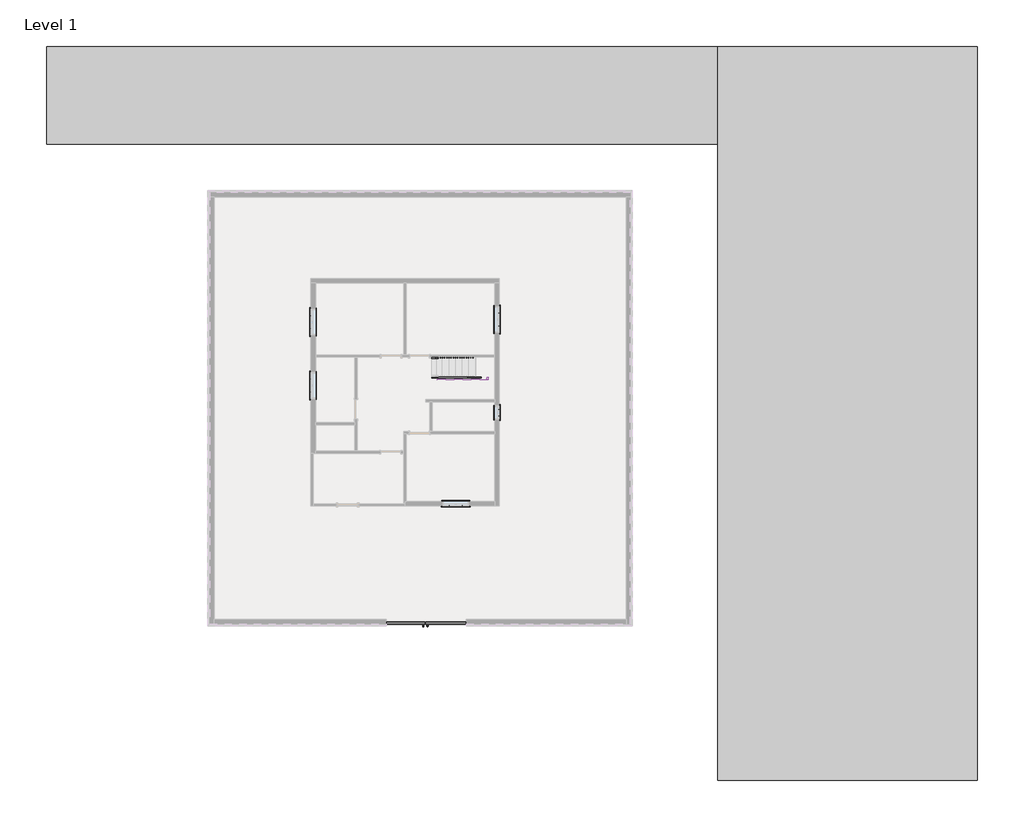
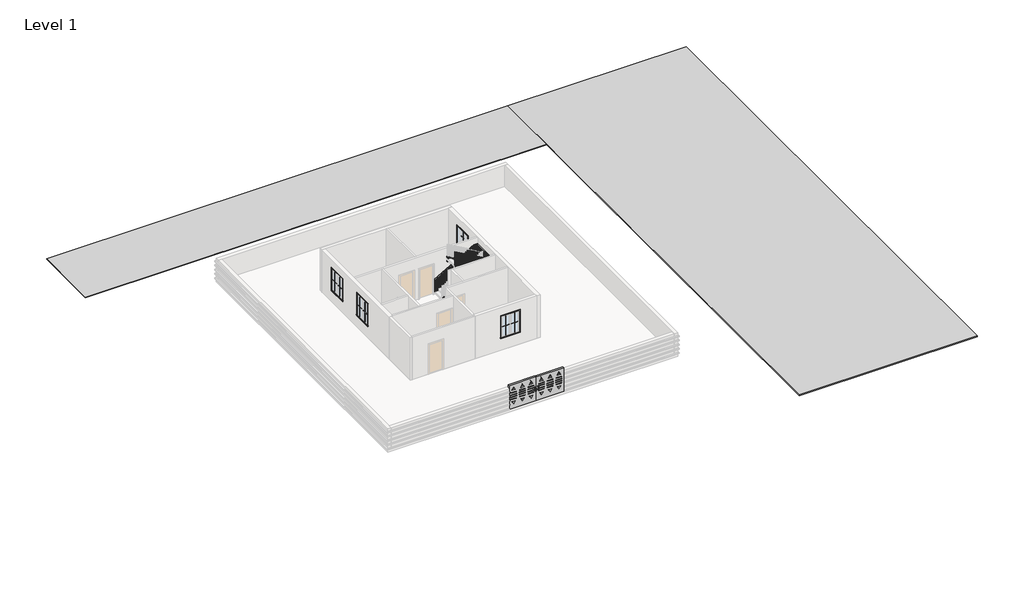
# One storey, part 3 of 3: 22 proxies, 3 members, 1 railing.
"""IFC4 building model written with IfcOpenShell, lengths in millimetres."""

from ifc_helpers import new_model, si_unit, frame, origin, place, context, project, spatial, polyline, outline, extrude, faceted_brep, transform, mapped, element, save
from components import generic_models_afecbd1f, generic_models_1_generic_models_1_28a2cc20, muntin_pattern_2x2_muntin_pattern_2x2_6dad3731, muntin_pattern_2x2_muntin_pattern_2x2_a30a3345, muntin_pattern_2x2_muntin_pattern_2x2_53152e2c, muntin_pattern_2x2_muntin_pattern_2x2_e8f3e573, trim_window_exterior_flat_with_sill_92b9b949, trim_window_exterior_flat_with_sill_a665a915, trim_window_interior_flat_picture_frame_3bb882cf, trim_window_interior_flat_picture_frame_d485c387

model = new_model("IFC4")

# Units and contexts
model_context = context("Model", 3, world=origin())
ifc_project = project(units=[si_unit("LENGTHUNIT", "METRE", prefix="MILLI")], contexts=[model_context])

# Site, building, storey
site = spatial("IfcSite", under=ifc_project)
building = spatial("IfcBuilding", under=site)
storey = spatial("IfcBuildingStorey", under=building, Name="Level 1", Elevation=0.0)

# Proxies
placement = place(None, origin())
generic_models_shape = generic_models_afecbd1f(model_context)
element("IfcBuildingElementProxy", 1, Name="Generic Models", at=placement, inside=storey, context=model_context, shape_type="MappedRepresentation", body=[
    mapped(generic_models_shape, transform((7975.8086384, -3206.75, 0.0), x_axis=(1.0, 0.0, 0.0), y_axis=(0.0, 1.0, 0.0), z_axis=(0.0, 0.0, 1.0))),
])
generic_models_1_generic_models_1_shape = generic_models_1_generic_models_1_28a2cc20(model_context)
element("IfcBuildingElementProxy", 2, Name="Generic Models 1 : Generic Models 1", ObjectType="Generic Models 1 : Generic Models 1", at=placement, inside=storey, context=model_context, shape_type="MappedRepresentation", body=[
    mapped(generic_models_1_generic_models_1_shape, transform((0.0, 0.0, 0.0), x_axis=(1.0, 0.0, 0.0), y_axis=(0.0, 1.0, 0.0), z_axis=(0.0, 0.0, 1.0))),
])
muntin_pattern_2x2_muntin_pattern_2x2_shape = muntin_pattern_2x2_muntin_pattern_2x2_6dad3731(model_context)
element("IfcBuildingElementProxy", 3, Name="Muntin Pattern_2x2 : Muntin Pattern_2x2", ObjectType="Muntin Pattern_2x2 : Muntin Pattern_2x2", at=placement, inside=storey, context=model_context, shape_type="MappedRepresentation", body=[
    mapped(muntin_pattern_2x2_muntin_pattern_2x2_shape, transform((10003.63125, 2232.025, 984.25), x_axis=(-1.0, 0.0, 0.0), y_axis=(0.0, -1.0, 0.0), z_axis=(0.0, 0.0, 1.0))),
])
element("IfcBuildingElementProxy", 4, Name="Muntin Pattern_2x2 : Muntin Pattern_2x2", ObjectType="Muntin Pattern_2x2 : Muntin Pattern_2x2", at=placement, inside=storey, context=model_context, shape_type="MappedRepresentation", body=[
    mapped(muntin_pattern_2x2_muntin_pattern_2x2_shape, transform((2917.825, 7567.6125, 984.25), x_axis=(0.0, 1.0, 0.0), y_axis=(-1.0, 0.0, 0.0), z_axis=(0.0, 0.0, 1.0))),
])
element("IfcBuildingElementProxy", 5, Name="Muntin Pattern_2x2 : Muntin Pattern_2x2", ObjectType="Muntin Pattern_2x2 : Muntin Pattern_2x2", at=placement, inside=storey, context=model_context, shape_type="MappedRepresentation", body=[
    mapped(muntin_pattern_2x2_muntin_pattern_2x2_shape, transform((2917.825, 10536.2375, 984.25), x_axis=(0.0, 1.0, 0.0), y_axis=(-1.0, 0.0, 0.0), z_axis=(0.0, 0.0, 1.0))),
])
element("IfcBuildingElementProxy", 6, Name="Muntin Pattern_2x2 : Muntin Pattern_2x2", ObjectType="Muntin Pattern_2x2 : Muntin Pattern_2x2", at=placement, inside=storey, context=model_context, shape_type="MappedRepresentation", body=[
    mapped(muntin_pattern_2x2_muntin_pattern_2x2_shape, transform((11737.975, 11264.9, 984.25), x_axis=(0.0, -1.0, 0.0), y_axis=(1.0, 0.0, 0.0), z_axis=(0.0, 0.0, 1.0))),
])
muntin_pattern_2x2_muntin_pattern_2x2_2_shape = muntin_pattern_2x2_muntin_pattern_2x2_a30a3345(model_context)
element("IfcBuildingElementProxy", 7, Name="Muntin Pattern_2x2 : Muntin Pattern_2x2", ObjectType="Muntin Pattern_2x2 : Muntin Pattern_2x2", at=placement, inside=storey, context=model_context, shape_type="MappedRepresentation", body=[
    mapped(muntin_pattern_2x2_muntin_pattern_2x2_2_shape, transform((9397.20625, 2232.025, 984.25), x_axis=(1.0, 0.0, 0.0), y_axis=(0.0, 1.0, 0.0), z_axis=(0.0, 0.0, 1.0))),
])
element("IfcBuildingElementProxy", 8, Name="Muntin Pattern_2x2 : Muntin Pattern_2x2", ObjectType="Muntin Pattern_2x2 : Muntin Pattern_2x2", at=placement, inside=storey, context=model_context, shape_type="MappedRepresentation", body=[
    mapped(muntin_pattern_2x2_muntin_pattern_2x2_2_shape, transform((2917.825, 8174.0375, 984.25), x_axis=(0.0, -1.0, 0.0), y_axis=(1.0, 0.0, 0.0), z_axis=(0.0, 0.0, 1.0))),
])
element("IfcBuildingElementProxy", 9, Name="Muntin Pattern_2x2 : Muntin Pattern_2x2", ObjectType="Muntin Pattern_2x2 : Muntin Pattern_2x2", at=placement, inside=storey, context=model_context, shape_type="MappedRepresentation", body=[
    mapped(muntin_pattern_2x2_muntin_pattern_2x2_2_shape, transform((2917.825, 11142.6625, 984.25), x_axis=(0.0, -1.0, 0.0), y_axis=(1.0, 0.0, 0.0), z_axis=(0.0, 0.0, 1.0))),
])
element("IfcBuildingElementProxy", 10, Name="Muntin Pattern_2x2 : Muntin Pattern_2x2", ObjectType="Muntin Pattern_2x2 : Muntin Pattern_2x2", at=placement, inside=storey, context=model_context, shape_type="MappedRepresentation", body=[
    mapped(muntin_pattern_2x2_muntin_pattern_2x2_2_shape, transform((11737.975, 10658.475, 984.25), x_axis=(0.0, 1.0, 0.0), y_axis=(-1.0, 0.0, 0.0), z_axis=(0.0, 0.0, 1.0))),
])
muntin_pattern_2x2_muntin_pattern_2x2_3_shape = muntin_pattern_2x2_muntin_pattern_2x2_53152e2c(model_context)
element("IfcBuildingElementProxy", 11, Name="Muntin Pattern_2x2 : Muntin Pattern_2x2", ObjectType="Muntin Pattern_2x2 : Muntin Pattern_2x2", at=placement, inside=storey, context=model_context, shape_type="MappedRepresentation", body=[
    mapped(muntin_pattern_2x2_muntin_pattern_2x2_3_shape, transform((11737.975, 6748.4625, 984.25), x_axis=(0.0, -1.0, 0.0), y_axis=(1.0, 0.0, 0.0), z_axis=(0.0, 0.0, 1.0))),
])
muntin_pattern_2x2_muntin_pattern_2x2_4_shape = muntin_pattern_2x2_muntin_pattern_2x2_e8f3e573(model_context)
element("IfcBuildingElementProxy", 12, Name="Muntin Pattern_2x2 : Muntin Pattern_2x2", ObjectType="Muntin Pattern_2x2 : Muntin Pattern_2x2", at=placement, inside=storey, context=model_context, shape_type="MappedRepresentation", body=[
    mapped(muntin_pattern_2x2_muntin_pattern_2x2_4_shape, transform((11737.975, 6446.8375, 984.25), x_axis=(0.0, 1.0, 0.0), y_axis=(-1.0, 0.0, 0.0), z_axis=(0.0, 0.0, 1.0))),
])
trim_window_exterior_flat_with_sill_shape = trim_window_exterior_flat_with_sill_92b9b949(model_context)
element("IfcBuildingElementProxy", 13, Name="Trim-Window-Exterior-Flat : with Sill", ObjectType="Trim-Window-Exterior-Flat : with Sill", at=placement, inside=storey, context=model_context, shape_type="MappedRepresentation", body=[
    mapped(trim_window_exterior_flat_with_sill_shape, transform((9700.41875, 2222.5, 2438.4), x_axis=(1.0, 0.0, 0.0), y_axis=(0.0, 0.0, 1.0), z_axis=(0.0, -1.0, 0.0))),
])
element("IfcBuildingElementProxy", 14, Name="Trim-Window-Exterior-Flat : with Sill", ObjectType="Trim-Window-Exterior-Flat : with Sill", at=placement, inside=storey, context=model_context, shape_type="MappedRepresentation", body=[
    mapped(trim_window_exterior_flat_with_sill_shape, transform((2908.3, 7870.825, 2438.4), x_axis=(0.0, -1.0, 0.0), y_axis=(0.0, 0.0, 1.0), z_axis=(-1.0, 0.0, 0.0))),
])
element("IfcBuildingElementProxy", 15, Name="Trim-Window-Exterior-Flat : with Sill", ObjectType="Trim-Window-Exterior-Flat : with Sill", at=placement, inside=storey, context=model_context, shape_type="MappedRepresentation", body=[
    mapped(trim_window_exterior_flat_with_sill_shape, transform((2908.3, 10839.45, 2438.4), x_axis=(0.0, -1.0, 0.0), y_axis=(0.0, 0.0, 1.0), z_axis=(-1.0, 0.0, 0.0))),
])
element("IfcBuildingElementProxy", 16, Name="Trim-Window-Exterior-Flat : with Sill", ObjectType="Trim-Window-Exterior-Flat : with Sill", at=placement, inside=storey, context=model_context, shape_type="MappedRepresentation", body=[
    mapped(trim_window_exterior_flat_with_sill_shape, transform((11747.5, 10961.6875, 2438.4), x_axis=(0.0, 1.0, 0.0), y_axis=(0.0, 0.0, 1.0), z_axis=(1.0, 0.0, 0.0))),
])
trim_window_exterior_flat_with_sill_2_shape = trim_window_exterior_flat_with_sill_a665a915(model_context)
element("IfcBuildingElementProxy", 17, Name="Trim-Window-Exterior-Flat : with Sill", ObjectType="Trim-Window-Exterior-Flat : with Sill", at=placement, inside=storey, context=model_context, shape_type="MappedRepresentation", body=[
    mapped(trim_window_exterior_flat_with_sill_2_shape, transform((11747.5, 6597.65, 1828.8), x_axis=(0.0, 1.0, 0.0), y_axis=(0.0, 0.0, 1.0), z_axis=(1.0, 0.0, 0.0))),
])
trim_window_interior_flat_picture_frame_shape = trim_window_interior_flat_picture_frame_3bb882cf(model_context)
element("IfcBuildingElementProxy", 18, Name="Trim-Window-Interior-Flat : Picture Frame", ObjectType="Trim-Window-Interior-Flat : Picture Frame", at=placement, inside=storey, context=model_context, shape_type="MappedRepresentation", body=[
    mapped(trim_window_interior_flat_picture_frame_shape, transform((9700.41875, 2451.1, 2438.4), x_axis=(-1.0, 0.0, 0.0), y_axis=(0.0, 0.0, 1.0), z_axis=(0.0, 1.0, 0.0))),
])
element("IfcBuildingElementProxy", 19, Name="Trim-Window-Interior-Flat : Picture Frame", ObjectType="Trim-Window-Interior-Flat : Picture Frame", at=placement, inside=storey, context=model_context, shape_type="MappedRepresentation", body=[
    mapped(trim_window_interior_flat_picture_frame_shape, transform((3136.9, 7870.825, 2438.4), x_axis=(0.0, 1.0, 0.0), y_axis=(0.0, 0.0, 1.0), z_axis=(1.0, 0.0, 0.0))),
])
element("IfcBuildingElementProxy", 20, Name="Trim-Window-Interior-Flat : Picture Frame", ObjectType="Trim-Window-Interior-Flat : Picture Frame", at=placement, inside=storey, context=model_context, shape_type="MappedRepresentation", body=[
    mapped(trim_window_interior_flat_picture_frame_shape, transform((3136.9, 10839.45, 2438.4), x_axis=(0.0, 1.0, 0.0), y_axis=(0.0, 0.0, 1.0), z_axis=(1.0, 0.0, 0.0))),
])
element("IfcBuildingElementProxy", 21, Name="Trim-Window-Interior-Flat : Picture Frame", ObjectType="Trim-Window-Interior-Flat : Picture Frame", at=placement, inside=storey, context=model_context, shape_type="MappedRepresentation", body=[
    mapped(trim_window_interior_flat_picture_frame_shape, transform((11518.9, 10961.6875, 2438.4), x_axis=(0.0, -1.0, 0.0), y_axis=(0.0, 0.0, 1.0), z_axis=(-1.0, 0.0, 0.0))),
])
trim_window_interior_flat_picture_frame_2_shape = trim_window_interior_flat_picture_frame_d485c387(model_context)
element("IfcBuildingElementProxy", 22, Name="Trim-Window-Interior-Flat : Picture Frame", ObjectType="Trim-Window-Interior-Flat : Picture Frame", at=placement, inside=storey, context=model_context, shape_type="MappedRepresentation", body=[
    mapped(trim_window_interior_flat_picture_frame_2_shape, transform((11518.9, 6597.65, 1828.8), x_axis=(0.0, -1.0, 0.0), y_axis=(0.0, 0.0, 1.0), z_axis=(-1.0, 0.0, 0.0))),
])

# Members
element("IfcMember", 23, ObjectType="Stringer - 2\" Width", at=placement, inside=storey, context=model_context, shape_type="SweptSolid", body=[
    extrude(outline(polyline([(249.0972589, 8572.5), (0.0, 8572.5), (0.0, 8751.427498), (1354.0336853, 11163.3), (1703.5814695, 11163.3), (249.0972589, 8572.5)])), frame((0.0, 8229.6, 0.0), z_axis=(0.0, 1.0, 0.0), x_axis=(0.0, 0.0, 1.0)), (0.0, 0.0, 1.0), 50.8),
])
element("IfcMember", 24, ObjectType="Stringer - 2\" Width", at=placement, inside=storey, context=model_context, shape_type="SweptSolid", body=[
    extrude(outline(polyline([(11163.3, 8280.4), (11214.1, 8280.4), (11214.1, 8178.8), (11163.3, 8178.8), (11163.3, 8280.4)])), frame((0.0, 0.0, 1464.7333333), z_axis=(0.0, 0.0, 1.0), x_axis=(1.0, 0.0, 0.0)), (0.0, 0.0, 1.0), 304.8),
])
element("IfcMember", 25, ObjectType="Stringer - 2\" Width", at=placement, inside=storey, context=model_context, shape_type="SweptSolid", body=[
    extrude(outline(polyline([(1552.253054, 11214.1), (1900.9317281, 11214.1), (3227.3761726, 8826.5), (2878.6974984, 8826.5), (1552.253054, 11214.1)])), frame((0.0, 8128.0, 0.0), z_axis=(0.0, 1.0, 0.0), x_axis=(0.0, 0.0, 1.0)), (0.0, 0.0, 1.0), 50.8),
])

# Railing
element("IfcRailing", 26, ObjectType="Handrail - Rectangular", at=placement, inside=storey, context=model_context, shape_type="SolidModel", body=[
    faceted_brep([(8572.5, 9194.8, 1083.7333333), (8572.5, 9194.8, 1025.0853937), (8572.5, 9144.0, 1025.0853937), (8572.5, 9144.0, 1083.7333333), (11214.1, 9194.8, 2607.7333333), (11227.7030954, 9194.8, 2556.9333333), (11227.7030954, 9144.0, 2556.9333333), (11214.1, 9144.0, 2607.7333333), (11518.9, 9194.8, 2607.7333333), (11518.9, 9194.8, 2556.9333333), (11468.1, 9144.0, 2556.9333333), (11468.1, 9144.0, 2607.7333333), (11518.9, 7340.6, 2607.7333333), (11518.9, 7289.8, 2556.9333333), (11468.1, 7289.8, 2556.9333333), (11468.1, 7340.6, 2607.7333333), (11518.9, 7340.6, 2676.187234), (11518.9, 7289.8, 2625.387234), (11468.1, 7289.8, 2625.387234), (11468.1, 7340.6, 2676.187234), (11518.9, 7213.6, 2676.187234), (11518.9, 7213.6, 2625.387234), (11468.1, 7264.4, 2625.387234), (11468.1, 7264.4, 2676.187234), (11391.9, 7213.6, 2676.187234), (11378.4925101, 7213.6, 2625.387234), (11378.4925101, 7264.4, 2625.387234), (11391.9, 7264.4, 2676.187234), (8826.5, 7213.6, 4131.7333333), (8826.5, 7264.4, 4131.7333333), (8826.5, 7264.4, 4073.3262469), (8826.5, 7213.6, 4073.3262469)], [[[0, 1, 2, 3]], [[1, 0, 4, 5]], [[2, 1, 5, 6]], [[3, 2, 6, 7]], [[0, 3, 7, 4]], [[5, 4, 8, 9]], [[6, 5, 9, 10]], [[7, 6, 10, 11]], [[4, 7, 11, 8]], [[9, 8, 12, 13]], [[10, 9, 13, 14]], [[11, 10, 14, 15]], [[8, 11, 15, 12]], [[13, 12, 16, 17]], [[14, 13, 17, 18]], [[15, 14, 18, 19]], [[12, 15, 19, 16]], [[17, 16, 20, 21]], [[18, 17, 21, 22]], [[19, 18, 22, 23]], [[16, 19, 23, 20]], [[21, 20, 24, 25]], [[22, 21, 25, 26]], [[23, 22, 26, 27]], [[20, 23, 27, 24]], [[28, 29, 30, 31]], [[25, 24, 28, 31]], [[26, 25, 31, 30]], [[27, 26, 30, 29]], [[24, 27, 29, 28]]]),
    extrude(outline(polyline([(4064.3191547, 8842.375), (3048.0, 8842.375), (3048.0, 8861.425), (4053.510644, 8861.425), (4064.3191547, 8842.375)])), frame((0.0, 7229.475, 0.0), z_axis=(0.0, 1.0, 0.0), x_axis=(0.0, 0.0, 1.0)), (0.0, 0.0, 1.0), 19.05),
    extrude(outline(polyline([(4006.6737646, 8943.975), (3048.0, 8943.975), (3048.0, 8963.025), (3995.865254, 8963.025), (4006.6737646, 8943.975)])), frame((0.0, 7229.475, 0.0), z_axis=(0.0, 1.0, 0.0), x_axis=(0.0, 0.0, 1.0)), (0.0, 0.0, 1.0), 19.05),
    extrude(outline(polyline([(3949.0283745, 9045.575), (3048.0, 9045.575), (3048.0, 9064.625), (3938.2198639, 9064.625), (3949.0283745, 9045.575)])), frame((0.0, 7229.475, 0.0), z_axis=(0.0, 1.0, 0.0), x_axis=(0.0, 0.0, 1.0)), (0.0, 0.0, 1.0), 19.05),
    extrude(outline(polyline([(3891.3829845, 9147.175), (2878.6666667, 9147.175), (2878.6666667, 9166.225), (3880.5744738, 9166.225), (3891.3829845, 9147.175)])), frame((0.0, 7229.475, 0.0), z_axis=(0.0, 1.0, 0.0), x_axis=(0.0, 0.0, 1.0)), (0.0, 0.0, 1.0), 19.05),
    extrude(outline(polyline([(3833.7375944, 9248.775), (2878.6666667, 9248.775), (2878.6666667, 9267.825), (3822.9290837, 9267.825), (3833.7375944, 9248.775)])), frame((0.0, 7229.475, 0.0), z_axis=(0.0, 1.0, 0.0), x_axis=(0.0, 0.0, 1.0)), (0.0, 0.0, 1.0), 19.05),
    extrude(outline(polyline([(3776.0922043, 9350.375), (2878.6666667, 9350.375), (2878.6666667, 9369.425), (3765.2836937, 9369.425), (3776.0922043, 9350.375)])), frame((0.0, 7229.475, 0.0), z_axis=(0.0, 1.0, 0.0), x_axis=(0.0, 0.0, 1.0)), (0.0, 0.0, 1.0), 19.05),
    extrude(outline(polyline([(3718.4468142, 9451.975), (2709.3333333, 9451.975), (2709.3333333, 9471.025), (3707.6383036, 9471.025), (3718.4468142, 9451.975)])), frame((0.0, 7229.475, 0.0), z_axis=(0.0, 1.0, 0.0), x_axis=(0.0, 0.0, 1.0)), (0.0, 0.0, 1.0), 19.05),
    extrude(outline(polyline([(3660.8014242, 9553.575), (2709.3333333, 9553.575), (2709.3333333, 9572.625), (3649.9929135, 9572.625), (3660.8014242, 9553.575)])), frame((0.0, 7229.475, 0.0), z_axis=(0.0, 1.0, 0.0), x_axis=(0.0, 0.0, 1.0)), (0.0, 0.0, 1.0), 19.05),
    extrude(outline(polyline([(3603.1446885, 9655.175), (2709.3333333, 9655.175), (2709.3333333, 9674.225), (3592.1543039, 9674.225), (3603.1446885, 9655.175)])), frame((0.0, 7229.475, 0.0), z_axis=(0.0, 1.0, 0.0), x_axis=(0.0, 0.0, 1.0)), (0.0, 0.0, 1.0), 19.05),
    extrude(outline(polyline([(3545.510644, 9756.775), (2540.0, 9756.775), (2540.0, 9775.825), (3534.7021334, 9775.825), (3545.510644, 9756.775)])), frame((0.0, 7229.475, 0.0), z_axis=(0.0, 1.0, 0.0), x_axis=(0.0, 0.0, 1.0)), (0.0, 0.0, 1.0), 19.05),
    extrude(outline(polyline([(3487.865254, 9858.375), (2540.0, 9858.375), (2540.0, 9877.425), (3477.0567433, 9877.425), (3487.865254, 9858.375)])), frame((0.0, 7229.475, 0.0), z_axis=(0.0, 1.0, 0.0), x_axis=(0.0, 0.0, 1.0)), (0.0, 0.0, 1.0), 19.05),
    extrude(outline(polyline([(3430.2198639, 9959.975), (2540.0, 9959.975), (2540.0, 9979.025), (3419.4113533, 9979.025), (3430.2198639, 9959.975)])), frame((0.0, 7229.475, 0.0), z_axis=(0.0, 1.0, 0.0), x_axis=(0.0, 0.0, 1.0)), (0.0, 0.0, 1.0), 19.05),
    extrude(outline(polyline([(3372.5744738, 10061.575), (2370.6666667, 10061.575), (2370.6666667, 10080.625), (3361.7659632, 10080.625), (3372.5744738, 10061.575)])), frame((0.0, 7229.475, 0.0), z_axis=(0.0, 1.0, 0.0), x_axis=(0.0, 0.0, 1.0)), (0.0, 0.0, 1.0), 19.05),
    extrude(outline(polyline([(3314.9290837, 10163.175), (2370.6666667, 10163.175), (2370.6666667, 10182.225), (3304.1205731, 10182.225), (3314.9290837, 10163.175)])), frame((0.0, 7229.475, 0.0), z_axis=(0.0, 1.0, 0.0), x_axis=(0.0, 0.0, 1.0)), (0.0, 0.0, 1.0), 19.05),
    extrude(outline(polyline([(3257.2836937, 10264.775), (2370.6666667, 10264.775), (2370.6666667, 10283.825), (3246.475183, 10283.825), (3257.2836937, 10264.775)])), frame((0.0, 7229.475, 0.0), z_axis=(0.0, 1.0, 0.0), x_axis=(0.0, 0.0, 1.0)), (0.0, 0.0, 1.0), 19.05),
    extrude(outline(polyline([(3199.6383036, 10366.375), (2201.3333333, 10366.375), (2201.3333333, 10385.425), (3188.829793, 10385.425), (3199.6383036, 10366.375)])), frame((0.0, 7229.475, 0.0), z_axis=(0.0, 1.0, 0.0), x_axis=(0.0, 0.0, 1.0)), (0.0, 0.0, 1.0), 19.05),
    extrude(outline(polyline([(3141.9929135, 10467.975), (2201.3333333, 10467.975), (2201.3333333, 10487.025), (3131.1844029, 10487.025), (3141.9929135, 10467.975)])), frame((0.0, 7229.475, 0.0), z_axis=(0.0, 1.0, 0.0), x_axis=(0.0, 0.0, 1.0)), (0.0, 0.0, 1.0), 19.05),
    extrude(outline(polyline([(3084.3475235, 10569.575), (2201.3333333, 10569.575), (2201.3333333, 10588.625), (3073.5390128, 10588.625), (3084.3475235, 10569.575)])), frame((0.0, 7229.475, 0.0), z_axis=(0.0, 1.0, 0.0), x_axis=(0.0, 0.0, 1.0)), (0.0, 0.0, 1.0), 19.05),
    extrude(outline(polyline([(3026.7021334, 10671.175), (2032.0, 10671.175), (2032.0, 10690.225), (3015.8936228, 10690.225), (3026.7021334, 10671.175)])), frame((0.0, 7229.475, 0.0), z_axis=(0.0, 1.0, 0.0), x_axis=(0.0, 0.0, 1.0)), (0.0, 0.0, 1.0), 19.05),
    extrude(outline(polyline([(2969.0567433, 10772.775), (2032.0, 10772.775), (2032.0, 10791.825), (2958.2482327, 10791.825), (2969.0567433, 10772.775)])), frame((0.0, 7229.475, 0.0), z_axis=(0.0, 1.0, 0.0), x_axis=(0.0, 0.0, 1.0)), (0.0, 0.0, 1.0), 19.05),
    extrude(outline(polyline([(2911.4113533, 10874.375), (2032.0, 10874.375), (2032.0, 10893.425), (2900.6028426, 10893.425), (2911.4113533, 10874.375)])), frame((0.0, 7229.475, 0.0), z_axis=(0.0, 1.0, 0.0), x_axis=(0.0, 0.0, 1.0)), (0.0, 0.0, 1.0), 19.05),
    extrude(outline(polyline([(2853.7659632, 10975.975), (1862.6666667, 10975.975), (1862.6666667, 10995.025), (2842.9574525, 10995.025), (2853.7659632, 10975.975)])), frame((0.0, 7229.475, 0.0), z_axis=(0.0, 1.0, 0.0), x_axis=(0.0, 0.0, 1.0)), (0.0, 0.0, 1.0), 19.05),
    extrude(outline(polyline([(2796.1205731, 11077.575), (1862.6666667, 11077.575), (1862.6666667, 11096.625), (2785.3120625, 11096.625), (2796.1205731, 11077.575)])), frame((0.0, 7229.475, 0.0), z_axis=(0.0, 1.0, 0.0), x_axis=(0.0, 0.0, 1.0)), (0.0, 0.0, 1.0), 19.05),
    extrude(outline(polyline([(2738.475183, 11179.175), (1862.6666667, 11179.175), (1862.6666667, 11198.225), (2727.6666724, 11198.225), (2738.475183, 11179.175)])), frame((0.0, 7229.475, 0.0), z_axis=(0.0, 1.0, 0.0), x_axis=(0.0, 0.0, 1.0)), (0.0, 0.0, 1.0), 19.05),
    extrude(outline(polyline([(2680.829793, 11280.775), (1693.3333333, 11280.775), (1693.3333333, 11299.825), (2670.0212823, 11299.825), (2680.829793, 11280.775)])), frame((0.0, 7229.475, 0.0), z_axis=(0.0, 1.0, 0.0), x_axis=(0.0, 0.0, 1.0)), (0.0, 0.0, 1.0), 19.05),
    extrude(outline(polyline([(2623.1844029, 11382.375), (1693.3333333, 11382.375), (1693.3333333, 11401.425), (2612.3758923, 11401.425), (2623.1844029, 11382.375)])), frame((0.0, 7229.475, 0.0), z_axis=(0.0, 1.0, 0.0), x_axis=(0.0, 0.0, 1.0)), (0.0, 0.0, 1.0), 19.05),
    extrude(outline(polyline([(11503.025, 7350.125), (11503.025, 7331.075), (11483.975, 7331.075), (11483.975, 7350.125), (11503.025, 7350.125)])), frame((0.0, 0.0, 1693.3333333), z_axis=(0.0, 0.0, 1.0), x_axis=(1.0, 0.0, 0.0)), (0.0, 0.0, 1.0), 863.6),
    extrude(outline(polyline([(11503.025, 7451.725), (11503.025, 7432.675), (11483.975, 7432.675), (11483.975, 7451.725), (11503.025, 7451.725)])), frame((0.0, 0.0, 1693.3333333), z_axis=(0.0, 0.0, 1.0), x_axis=(1.0, 0.0, 0.0)), (0.0, 0.0, 1.0), 863.6),
    extrude(outline(polyline([(11503.025, 7553.325), (11503.025, 7534.275), (11483.975, 7534.275), (11483.975, 7553.325), (11503.025, 7553.325)])), frame((0.0, 0.0, 1693.3333333), z_axis=(0.0, 0.0, 1.0), x_axis=(1.0, 0.0, 0.0)), (0.0, 0.0, 1.0), 863.6),
    extrude(outline(polyline([(11503.025, 7654.925), (11503.025, 7635.875), (11483.975, 7635.875), (11483.975, 7654.925), (11503.025, 7654.925)])), frame((0.0, 0.0, 1693.3333333), z_axis=(0.0, 0.0, 1.0), x_axis=(1.0, 0.0, 0.0)), (0.0, 0.0, 1.0), 863.6),
    extrude(outline(polyline([(11503.025, 7756.525), (11503.025, 7737.475), (11483.975, 7737.475), (11483.975, 7756.525), (11503.025, 7756.525)])), frame((0.0, 0.0, 1693.3333333), z_axis=(0.0, 0.0, 1.0), x_axis=(1.0, 0.0, 0.0)), (0.0, 0.0, 1.0), 863.6),
    extrude(outline(polyline([(11503.025, 7858.125), (11503.025, 7839.075), (11483.975, 7839.075), (11483.975, 7858.125), (11503.025, 7858.125)])), frame((0.0, 0.0, 1693.3333333), z_axis=(0.0, 0.0, 1.0), x_axis=(1.0, 0.0, 0.0)), (0.0, 0.0, 1.0), 863.6),
    extrude(outline(polyline([(11503.025, 7959.725), (11503.025, 7940.675), (11483.975, 7940.675), (11483.975, 7959.725), (11503.025, 7959.725)])), frame((0.0, 0.0, 1693.3333333), z_axis=(0.0, 0.0, 1.0), x_axis=(1.0, 0.0, 0.0)), (0.0, 0.0, 1.0), 863.6),
    extrude(outline(polyline([(11503.025, 8061.325), (11503.025, 8042.275), (11483.975, 8042.275), (11483.975, 8061.325), (11503.025, 8061.325)])), frame((0.0, 0.0, 1693.3333333), z_axis=(0.0, 0.0, 1.0), x_axis=(1.0, 0.0, 0.0)), (0.0, 0.0, 1.0), 863.6),
    extrude(outline(polyline([(11503.025, 8162.925), (11503.025, 8143.875), (11483.975, 8143.875), (11483.975, 8162.925), (11503.025, 8162.925)])), frame((0.0, 0.0, 1693.3333333), z_axis=(0.0, 0.0, 1.0), x_axis=(1.0, 0.0, 0.0)), (0.0, 0.0, 1.0), 863.6),
    extrude(outline(polyline([(11503.025, 8264.525), (11503.025, 8245.475), (11483.975, 8245.475), (11483.975, 8264.525), (11503.025, 8264.525)])), frame((0.0, 0.0, 1693.3333333), z_axis=(0.0, 0.0, 1.0), x_axis=(1.0, 0.0, 0.0)), (0.0, 0.0, 1.0), 863.6),
    extrude(outline(polyline([(11503.025, 8366.125), (11503.025, 8347.075), (11483.975, 8347.075), (11483.975, 8366.125), (11503.025, 8366.125)])), frame((0.0, 0.0, 1693.3333333), z_axis=(0.0, 0.0, 1.0), x_axis=(1.0, 0.0, 0.0)), (0.0, 0.0, 1.0), 863.6),
    extrude(outline(polyline([(11503.025, 8467.725), (11503.025, 8448.675), (11483.975, 8448.675), (11483.975, 8467.725), (11503.025, 8467.725)])), frame((0.0, 0.0, 1693.3333333), z_axis=(0.0, 0.0, 1.0), x_axis=(1.0, 0.0, 0.0)), (0.0, 0.0, 1.0), 863.6),
    extrude(outline(polyline([(11503.025, 8569.325), (11503.025, 8550.275), (11483.975, 8550.275), (11483.975, 8569.325), (11503.025, 8569.325)])), frame((0.0, 0.0, 1693.3333333), z_axis=(0.0, 0.0, 1.0), x_axis=(1.0, 0.0, 0.0)), (0.0, 0.0, 1.0), 863.6),
    extrude(outline(polyline([(11503.025, 8670.925), (11503.025, 8651.875), (11483.975, 8651.875), (11483.975, 8670.925), (11503.025, 8670.925)])), frame((0.0, 0.0, 1693.3333333), z_axis=(0.0, 0.0, 1.0), x_axis=(1.0, 0.0, 0.0)), (0.0, 0.0, 1.0), 863.6),
    extrude(outline(polyline([(11503.025, 8772.525), (11503.025, 8753.475), (11483.975, 8753.475), (11483.975, 8772.525), (11503.025, 8772.525)])), frame((0.0, 0.0, 1693.3333333), z_axis=(0.0, 0.0, 1.0), x_axis=(1.0, 0.0, 0.0)), (0.0, 0.0, 1.0), 863.6),
    extrude(outline(polyline([(11503.025, 8874.125), (11503.025, 8855.075), (11483.975, 8855.075), (11483.975, 8874.125), (11503.025, 8874.125)])), frame((0.0, 0.0, 1693.3333333), z_axis=(0.0, 0.0, 1.0), x_axis=(1.0, 0.0, 0.0)), (0.0, 0.0, 1.0), 863.6),
    extrude(outline(polyline([(11503.025, 8975.725), (11503.025, 8956.675), (11483.975, 8956.675), (11483.975, 8975.725), (11503.025, 8975.725)])), frame((0.0, 0.0, 1693.3333333), z_axis=(0.0, 0.0, 1.0), x_axis=(1.0, 0.0, 0.0)), (0.0, 0.0, 1.0), 863.6),
    extrude(outline(polyline([(11503.025, 9077.325), (11503.025, 9058.275), (11483.975, 9058.275), (11483.975, 9077.325), (11503.025, 9077.325)])), frame((0.0, 0.0, 1693.3333333), z_axis=(0.0, 0.0, 1.0), x_axis=(1.0, 0.0, 0.0)), (0.0, 0.0, 1.0), 863.6),
    extrude(outline(polyline([(11407.775, 9178.925), (11426.825, 9178.925), (11426.825, 9159.875), (11407.775, 9159.875), (11407.775, 9178.925)])), frame((0.0, 0.0, 1693.3333333), z_axis=(0.0, 0.0, 1.0), x_axis=(1.0, 0.0, 0.0)), (0.0, 0.0, 1.0), 863.6),
    extrude(outline(polyline([(11306.175, 9178.925), (11325.225, 9178.925), (11325.225, 9159.875), (11306.175, 9159.875), (11306.175, 9178.925)])), frame((0.0, 0.0, 1693.3333333), z_axis=(0.0, 0.0, 1.0), x_axis=(1.0, 0.0, 0.0)), (0.0, 0.0, 1.0), 863.6),
    extrude(outline(polyline([(2543.5902013, 11204.575), (1693.3333333, 11204.575), (1693.3333333, 11223.625), (2554.580586, 11223.625), (2543.5902013, 11204.575)])), frame((0.0, 9159.875, 0.0), z_axis=(0.0, 1.0, 0.0), x_axis=(0.0, 0.0, 1.0)), (0.0, 0.0, 1.0), 19.05),
    extrude(outline(polyline([(2484.9748167, 11102.975), (1524.0, 11102.975), (1524.0, 11122.025), (2495.9652013, 11122.025), (2484.9748167, 11102.975)])), frame((0.0, 9159.875, 0.0), z_axis=(0.0, 1.0, 0.0), x_axis=(0.0, 0.0, 1.0)), (0.0, 0.0, 1.0), 19.05),
    extrude(outline(polyline([(2426.3594321, 11001.375), (1524.0, 11001.375), (1524.0, 11020.425), (2437.3498167, 11020.425), (2426.3594321, 11001.375)])), frame((0.0, 9159.875, 0.0), z_axis=(0.0, 1.0, 0.0), x_axis=(0.0, 0.0, 1.0)), (0.0, 0.0, 1.0), 19.05),
    extrude(outline(polyline([(2367.7440475, 10899.775), (1524.0, 10899.775), (1524.0, 10918.825), (2378.7344321, 10918.825), (2367.7440475, 10899.775)])), frame((0.0, 9159.875, 0.0), z_axis=(0.0, 1.0, 0.0), x_axis=(0.0, 0.0, 1.0)), (0.0, 0.0, 1.0), 19.05),
    extrude(outline(polyline([(2309.1286629, 10798.175), (1354.6666667, 10798.175), (1354.6666667, 10817.225), (2320.1190475, 10817.225), (2309.1286629, 10798.175)])), frame((0.0, 9159.875, 0.0), z_axis=(0.0, 1.0, 0.0), x_axis=(0.0, 0.0, 1.0)), (0.0, 0.0, 1.0), 19.05),
    extrude(outline(polyline([(2250.5132783, 10696.575), (1354.6666667, 10696.575), (1354.6666667, 10715.625), (2261.5036629, 10715.625), (2250.5132783, 10696.575)])), frame((0.0, 9159.875, 0.0), z_axis=(0.0, 1.0, 0.0), x_axis=(0.0, 0.0, 1.0)), (0.0, 0.0, 1.0), 19.05),
    extrude(outline(polyline([(2191.8978937, 10594.975), (1354.6666667, 10594.975), (1354.6666667, 10614.025), (2202.8882783, 10614.025), (2191.8978937, 10594.975)])), frame((0.0, 9159.875, 0.0), z_axis=(0.0, 1.0, 0.0), x_axis=(0.0, 0.0, 1.0)), (0.0, 0.0, 1.0), 19.05),
    extrude(outline(polyline([(2133.282509, 10493.375), (1185.3333333, 10493.375), (1185.3333333, 10512.425), (2144.2728937, 10512.425), (2133.282509, 10493.375)])), frame((0.0, 9159.875, 0.0), z_axis=(0.0, 1.0, 0.0), x_axis=(0.0, 0.0, 1.0)), (0.0, 0.0, 1.0), 19.05),
    extrude(outline(polyline([(2074.6671244, 10391.775), (1185.3333333, 10391.775), (1185.3333333, 10410.825), (2085.657509, 10410.825), (2074.6671244, 10391.775)])), frame((0.0, 9159.875, 0.0), z_axis=(0.0, 1.0, 0.0), x_axis=(0.0, 0.0, 1.0)), (0.0, 0.0, 1.0), 19.05),
    extrude(outline(polyline([(2016.0517398, 10290.175), (1185.3333333, 10290.175), (1185.3333333, 10309.225), (2027.0421244, 10309.225), (2016.0517398, 10290.175)])), frame((0.0, 9159.875, 0.0), z_axis=(0.0, 1.0, 0.0), x_axis=(0.0, 0.0, 1.0)), (0.0, 0.0, 1.0), 19.05),
    extrude(outline(polyline([(1957.4363552, 10188.575), (1016.0, 10188.575), (1016.0, 10207.625), (1968.4267398, 10207.625), (1957.4363552, 10188.575)])), frame((0.0, 9159.875, 0.0), z_axis=(0.0, 1.0, 0.0), x_axis=(0.0, 0.0, 1.0)), (0.0, 0.0, 1.0), 19.05),
    extrude(outline(polyline([(1898.8209706, 10086.975), (1016.0, 10086.975), (1016.0, 10106.025), (1909.8113552, 10106.025), (1898.8209706, 10086.975)])), frame((0.0, 9159.875, 0.0), z_axis=(0.0, 1.0, 0.0), x_axis=(0.0, 0.0, 1.0)), (0.0, 0.0, 1.0), 19.05),
    extrude(outline(polyline([(1840.205586, 9985.375), (1016.0, 9985.375), (1016.0, 10004.425), (1851.1959706, 10004.425), (1840.205586, 9985.375)])), frame((0.0, 9159.875, 0.0), z_axis=(0.0, 1.0, 0.0), x_axis=(0.0, 0.0, 1.0)), (0.0, 0.0, 1.0), 19.05),
    extrude(outline(polyline([(1781.5902013, 9883.775), (846.6666667, 9883.775), (846.6666667, 9902.825), (1792.580586, 9902.825), (1781.5902013, 9883.775)])), frame((0.0, 9159.875, 0.0), z_axis=(0.0, 1.0, 0.0), x_axis=(0.0, 0.0, 1.0)), (0.0, 0.0, 1.0), 19.05),
    extrude(outline(polyline([(1722.9748167, 9782.175), (846.6666667, 9782.175), (846.6666667, 9801.225), (1733.9652013, 9801.225), (1722.9748167, 9782.175)])), frame((0.0, 9159.875, 0.0), z_axis=(0.0, 1.0, 0.0), x_axis=(0.0, 0.0, 1.0)), (0.0, 0.0, 1.0), 19.05),
    extrude(outline(polyline([(1664.3594321, 9680.575), (846.6666667, 9680.575), (846.6666667, 9699.625), (1675.3498167, 9699.625), (1664.3594321, 9680.575)])), frame((0.0, 9159.875, 0.0), z_axis=(0.0, 1.0, 0.0), x_axis=(0.0, 0.0, 1.0)), (0.0, 0.0, 1.0), 19.05),
    extrude(outline(polyline([(1605.7440475, 9578.975), (677.3333333, 9578.975), (677.3333333, 9598.025), (1616.7344321, 9598.025), (1605.7440475, 9578.975)])), frame((0.0, 9159.875, 0.0), z_axis=(0.0, 1.0, 0.0), x_axis=(0.0, 0.0, 1.0)), (0.0, 0.0, 1.0), 19.05),
    extrude(outline(polyline([(1547.1286629, 9477.375), (677.3333333, 9477.375), (677.3333333, 9496.425), (1558.1190475, 9496.425), (1547.1286629, 9477.375)])), frame((0.0, 9159.875, 0.0), z_axis=(0.0, 1.0, 0.0), x_axis=(0.0, 0.0, 1.0)), (0.0, 0.0, 1.0), 19.05),
    extrude(outline(polyline([(1488.5132783, 9375.775), (677.3333333, 9375.775), (677.3333333, 9394.825), (1499.5036629, 9394.825), (1488.5132783, 9375.775)])), frame((0.0, 9159.875, 0.0), z_axis=(0.0, 1.0, 0.0), x_axis=(0.0, 0.0, 1.0)), (0.0, 0.0, 1.0), 19.05),
    extrude(outline(polyline([(1429.8978937, 9274.175), (508.0, 9274.175), (508.0, 9293.225), (1440.8882783, 9293.225), (1429.8978937, 9274.175)])), frame((0.0, 9159.875, 0.0), z_axis=(0.0, 1.0, 0.0), x_axis=(0.0, 0.0, 1.0)), (0.0, 0.0, 1.0), 19.05),
    extrude(outline(polyline([(1371.282509, 9172.575), (508.0, 9172.575), (508.0, 9191.625), (1382.2728937, 9191.625), (1371.282509, 9172.575)])), frame((0.0, 9159.875, 0.0), z_axis=(0.0, 1.0, 0.0), x_axis=(0.0, 0.0, 1.0)), (0.0, 0.0, 1.0), 19.05),
    extrude(outline(polyline([(1312.6671244, 9070.975), (508.0, 9070.975), (508.0, 9090.025), (1323.657509, 9090.025), (1312.6671244, 9070.975)])), frame((0.0, 9159.875, 0.0), z_axis=(0.0, 1.0, 0.0), x_axis=(0.0, 0.0, 1.0)), (0.0, 0.0, 1.0), 19.05),
    extrude(outline(polyline([(1254.0517398, 8969.375), (338.6666667, 8969.375), (338.6666667, 8988.425), (1265.0421244, 8988.425), (1254.0517398, 8969.375)])), frame((0.0, 9159.875, 0.0), z_axis=(0.0, 1.0, 0.0), x_axis=(0.0, 0.0, 1.0)), (0.0, 0.0, 1.0), 19.05),
    extrude(outline(polyline([(1195.4363552, 8867.775), (338.6666667, 8867.775), (338.6666667, 8886.825), (1206.4267398, 8886.825), (1195.4363552, 8867.775)])), frame((0.0, 9159.875, 0.0), z_axis=(0.0, 1.0, 0.0), x_axis=(0.0, 0.0, 1.0)), (0.0, 0.0, 1.0), 19.05),
    extrude(outline(polyline([(1136.8209706, 8766.175), (169.3333333, 8766.175), (169.3333333, 8785.225), (1147.8113552, 8785.225), (1136.8209706, 8766.175)])), frame((0.0, 9159.875, 0.0), z_axis=(0.0, 1.0, 0.0), x_axis=(0.0, 0.0, 1.0)), (0.0, 0.0, 1.0), 19.05),
    extrude(outline(polyline([(1078.205586, 8664.575), (169.3333333, 8664.575), (169.3333333, 8683.625), (1089.1959706, 8683.625), (1078.205586, 8664.575)])), frame((0.0, 9159.875, 0.0), z_axis=(0.0, 1.0, 0.0), x_axis=(0.0, 0.0, 1.0)), (0.0, 0.0, 1.0), 19.05),
    extrude(outline(polyline([(11503.025, 7248.525), (11503.025, 7229.475), (11483.975, 7229.475), (11483.975, 7248.525), (11503.025, 7248.525)])), frame((0.0, 0.0, 1693.3333333), z_axis=(0.0, 0.0, 1.0), x_axis=(1.0, 0.0, 0.0)), (0.0, 0.0, 1.0), 932.0539007),
    extrude(outline(polyline([(11483.975, 9178.925), (11503.025, 9178.925), (11503.025, 9159.875), (11483.975, 9159.875), (11483.975, 9178.925)])), frame((0.0, 0.0, 1693.3333333), z_axis=(0.0, 0.0, 1.0), x_axis=(1.0, 0.0, 0.0)), (0.0, 0.0, 1.0), 863.6),
    extrude(outline(polyline([(4073.3262469, 8826.5), (3048.0, 8826.5), (3048.0, 8845.55), (4062.5177362, 8845.55), (4073.3262469, 8826.5)])), frame((0.0, 7229.475, 0.0), z_axis=(0.0, 1.0, 0.0), x_axis=(0.0, 0.0, 1.0)), (0.0, 0.0, 1.0), 19.05),
    extrude(outline(polyline([(1025.0853937, 8572.5), (169.3333333, 8572.5), (169.3333333, 8591.55), (1036.0757783, 8591.55), (1025.0853937, 8572.5)])), frame((0.0, 9159.875, 0.0), z_axis=(0.0, 1.0, 0.0), x_axis=(0.0, 0.0, 1.0)), (0.0, 0.0, 1.0), 19.05),
])

save(model, "model.ifc")

# Revit data of these elements
# Type
#   Default Elevation = 0
# Type "Muntin Pattern_2x2 : Muntin Pattern_2x2"
#   Width [instance default] = 4' - 0"
#   Thickness = 0' - 0 1/2"
#   Height [instance default] = 4' - 0"
#   Distance = 0' - 0 3/4"
#   Interior Material [instance default] = none
#   Exterior Material [instance default] = none
#   Default Elevation = 0
# Type "Trim-Window-Exterior-Flat : with Sill"
#   Trim Width = 0' - 2 1/4"
#   Trim Thickness_Picture Frame = 0' - 1 1/4"
#   Trim Thickness_with Sill = 0' - 0 3/4"
#   Sill Thickness = 0' - 1 1/4"
#   Opening Width [instance default] = 2' - 0"
#   Opening Height [instance default] = 3' - 0"
#   Default Elevation = 4' - 0"
#   Sill = yes
#   Picture Frame = no
#   Trim Material [instance default] = none
# Type "Trim-Window-Interior-Flat : Picture Frame"
#   Trim Thickness_Picture Frame = 0' - 1 1/4"
#   Trim Width = 0' - 2 1/4"
#   Trim Thickness_with Sill = 0' - 0 3/4"
#   Sill Thickness = 0' - 1 1/4"
#   Opening Width [instance default] = 2' - 0"
#   Opening Height [instance default] = 3' - 0"
#   Default Elevation = 4' - 0"
#   Sill = no
#   Picture Frame = yes
#   Trim Material [instance default] = none
# Type "Handrail - Rectangular"
#   Assembly Code = "C2010400"
#   built-in parameter 1008612 = 0.0416667 (stored number, unit not read)
#   built-in parameter 1008611 = 0.0416667 (stored number, unit not read)
#   built-in parameter 1008609 = 0.333333 (stored number, unit not read)
#   built-in parameter 1008604 = 0.166667 (stored number, unit not read)
#   built-in parameter 1008603 = 0.166667 (stored number, unit not read)
#   Railing Height = 3' - 0"
#   built-in parameter 1008630 = 2
#   built-in parameter 1008610 = 2
#   built-in parameter 1008618 = Baluster - Square : 3/4"
# Element 1 (IfcBuildingElementProxy)
#   Phase Created = New Construction
#   Materials on its faces: "GATE"
# Element 2 (IfcBuildingElementProxy, "Generic Models 1 : Generic Models 1")
#   Phase Created = New Construction
# Elements 3, 4, 5, 6, 7, 8, 9, 10 (IfcBuildingElementProxy, "Muntin Pattern_2x2 : Muntin Pattern_2x2")
#   Width = 1' - 6 5/8"
#   Height = 4' - 6 1/2"
#   Interior Material = Wood - Stained
#   Exterior Material = Clad - White
#   Phase Created = New Construction
#   Materials on its faces: "Clad - White", "Wood - Stained"
# Elements 11, 12 (IfcBuildingElementProxy, "Muntin Pattern_2x2 : Muntin Pattern_2x2")
#   Width = 0' - 6 5/8"
#   Height = 2' - 6 1/2"
#   Interior Material = Wood - Stained
#   Exterior Material = Clad - White
#   Phase Created = New Construction
#   Materials on its faces: "Clad - White", "Wood - Stained"
# Elements 13, 14, 15, 16 (IfcBuildingElementProxy, "Trim-Window-Exterior-Flat : with Sill")
#   Opening Width = 4' - 0"
#   Opening Height = 5' - 0"
#   Trim Material = Clad - White
#   Phase Created = New Construction
#   Materials on its faces: "Clad - White"
# Element 17 (IfcBuildingElementProxy, "Trim-Window-Exterior-Flat : with Sill")
#   Opening Width = 2' - 0"
#   Opening Height = 3' - 0"
#   Trim Material = Clad - White
#   Phase Created = New Construction
#   Materials on its faces: "Clad - White"
# Elements 18, 19, 20, 21 (IfcBuildingElementProxy, "Trim-Window-Interior-Flat : Picture Frame")
#   Opening Width = 4' - 0"
#   Opening Height = 5' - 0"
#   Trim Material = Wood - Stained
#   Phase Created = New Construction
#   Materials on its faces: "Wood - Stained"
# Element 22 (IfcBuildingElementProxy, "Trim-Window-Interior-Flat : Picture Frame")
#   Opening Width = 2' - 0"
#   Opening Height = 3' - 0"
#   Trim Material = Wood - Stained
#   Phase Created = New Construction
#   Materials on its faces: "Wood - Stained"
# Elements 23, 24, 25 (IfcMember, "Stringer - 2\" Width")
#   Phase Created = New Construction
# Element 26 (IfcRailing, "Handrail - Rectangular")
#   Phase Created = New Construction
# Materials
#   "GATE": class "Generic", colour RGB 120 120 120, transparency 0, Cost = 0
#   "Clad - White": class "Wood", colour RGB 242 242 238, transparency 0, Cost = 0
#   "Wood - Stained": class "Wood", colour RGB 224 178 126, transparency 0, Cost = 0
